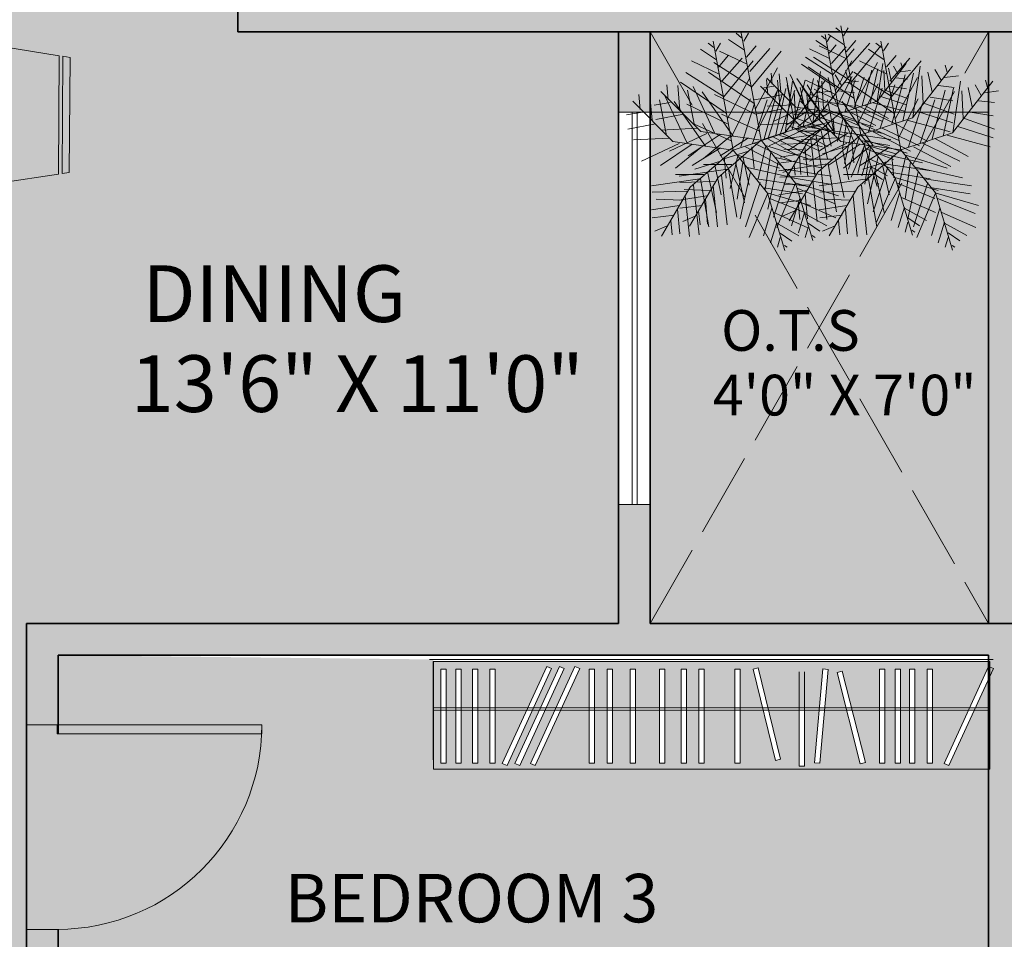
# Model space of a CAD drawing. Units: inches. Extents: x 1316 to 1777, y 813 to 1650.
# Tile 15 of 22: x 1567 to 1706, y 1237 to 1367. Entities that reach past the tile are written whole.
import ezdxf

# ---------------------------------------------------------------- set-up
doc = ezdxf.new("R2010")
doc.units = ezdxf.units.IN
doc.header["$MEASUREMENT"] = 0
doc.linetypes.add('ACAD_ISO02W100', pattern=[15, 12, -3])
for name, color, linetype, lineweight in [('A-AREA-IDEN', 7, 'Continuous', 18), ('A-DOOR', 4, 'Continuous', 18), ('A-DOOR-PATT', 253, 'Continuous', 13), ('A-FLOR-CASE-PATT', 252, 'Continuous', 13), ('A-FLOR-OPEN', 8, 'ACAD_ISO02W100', 13), ('A-FURN-PATT', 23, 'Continuous', 13), ('A-WALL-PATT', 250, 'Continuous', 13), ('closet', 23, 'Continuous', 18), ('furniture', 23, 'Continuous', 18), ('greenary', 106, 'Continuous', 13), ('L-HRDS', 8, 'Continuous', 18), ('L-HRDS-PATT', 252, 'Continuous', 13), ('L-PLNT-PATT', 74, 'Continuous', 13), ('walls', 250, 'Continuous', 35), ('windows', 141, 'Continuous', 18)]:
    doc.layers.add(name, color=color, linetype=linetype, lineweight=lineweight)
doc.layers.add('A-FLOR-PATT', color=254, linetype='Continuous', lineweight=13, true_color=0xfeeab9)
doc.styles.get("Standard").update_dxf_attribs({"font": 'arial.ttf'})

# ---------------------------------------------------------------- blocks, each defined once
blk = doc.blocks.new('*U15')
for p, q in [((0, 0), (0, -6)), ((40, 0), (40, -6))]:
    blk.add_line(p, q)
blk.add_lwpolyline([(0, 0), (0, 40), (1.75, 40), (1.75, 0)], close=True)
blk.add_arc((0, 0), 40, 0, 90)
blk = doc.blocks.new('Dining Set - 36 x 72 in.')
for p, q in [((-22, 27.5), (-22.1562, 26.50042)), ((-22, 27.5), (-6, 27.5)), ((-5.8437, 26.49966), (-6, 27.5)), ((6, 27.5), (5.8438, 26.50042)), ((6, 27.5), (22, 27.5)), ((22.1563, 26.49966), (22, 27.5)), ((-5.8416, 26.5), (-22.1534, 26.5)), ((22.1584, 26.5), (5.8466, 26.5)), ((-22.2343, 26.00059), (-23.4847, 17.99762)), ((-22.2304, 26), (-5.7608, 26)), ((-4.5152, 17.99762), (-5.7655, 25.99926)), ((5.7657, 26.00059), (4.5153, 17.99762)), ((5.7696, 26), (22.2392, 26)), ((23.4848, 17.99762), (22.2345, 25.99926)), ((36, 18), (-36, 18)), ((-36, 18), (-36, -18)), ((36, -18), (36, 18)), ((-44.0006, 8.23428), (-35.9976, 9.48474)), ((-44, 8.23041), (-44, -8.23915)), ((44.0006, 8.23428), (35.9976, 9.48474)), ((44, 8.23041), (44, -8.23915)), ((-45.5, 8), (-44.5004, 8.15617)), ((-45.5, 8), (-45.5, -8)), ((-44.5, -8.15843), (-44.5, 8.15338)), ((44.5, -8.15843), (44.5, 8.15338)), ((45.5, 8), (44.5005, 8.15617)), ((45.5, 8), (45.5, -8)), ((-44.4997, -8.15631), (-45.5, -8)), ((44.4997, -8.15631), (45.5, -8)), ((-35.9976, -9.48476), (-43.9993, -8.2345)), ((35.9976, -9.48476), (43.9993, -8.2345)), ((-36, -18), (36, -18)), ((-22.2343, -26.0006), (-23.4847, -17.99762)), ((-4.5152, -17.99762), (-5.7655, -25.99928)), ((5.7657, -26.0006), (4.5153, -17.99762)), ((23.4848, -17.99762), (22.2345, -25.99928)), ((-22.2304, -26), (-5.7608, -26)), ((5.7696, -26), (22.2392, -26)), ((-22, -27.5), (-22.1562, -26.50044)), ((-5.8416, -26.5), (-22.1534, -26.5)), ((-5.8437, -26.49967), (-6, -27.5)), ((6, -27.5), (5.8438, -26.50044)), ((22.1584, -26.5), (5.8466, -26.5)), ((22.1563, -26.49967), (22, -27.5)), ((-22, -27.5), (-6, -27.5)), ((6, -27.5), (22, -27.5))]:
    blk.add_line(p, q)
for points in [[(-36, 15), (-31.1772, 14.97754), (-26.8079, 14.91406), (-22.8538, 14.81543), (-19.276, 14.6875), (-16.0362, 14.53613), (-13.0957, 14.36718), (-10.4159, 14.18652), (-7.9583, 14), (-5.6904, 13.81315), (-3.6035, 13.63021), (-1.6954, 13.45508), (0.0365, 13.29166), (1.5945, 13.14388), (2.9811, 13.01562), (4.1988, 12.9108), (5.25, 12.83333), (6.1393, 12.78613), (6.8802, 12.76823), (7.4883, 12.77767), (7.9792, 12.8125), (8.3685, 12.87077), (8.6719, 12.95052), (8.9049, 13.0498), (9.0833, 13.16666), (9.2205, 13.29899), (9.3216, 13.44401), (9.3895, 13.59879), (9.4271, 13.76041), (9.4373, 13.92594), (9.4232, 14.09245), (9.3875, 14.257), (9.3333, 14.41666), (9.2638, 14.56917), (9.1836, 14.71484), (9.0975, 14.85465), (9.0104, 14.98958), (8.9272, 15.1206), (8.8529, 15.2487), (8.7922, 15.37483), (8.75, 15.5), (8.7305, 15.62467), (8.7344, 15.74739), (8.7617, 15.86621), (8.8125, 15.97916), (8.8867, 16.08431), (8.9844, 16.17968), (9.1055, 16.26334), (9.25, 16.33333), (9.4189, 16.38802), (9.6172, 16.42708), (9.8506, 16.45052), (10.125, 16.45833), (10.4463, 16.45052), (10.8203, 16.42708), (11.2529, 16.38802), (11.75, 16.33333), (12.3184, 16.26318), (12.9694, 16.17838), (13.7151, 16.07991), (14.5677, 15.96875), (15.5395, 15.84586), (16.6426, 15.71224), (17.8893, 15.56884), (19.2917, 15.41666), (20.859, 15.25667), (22.5879, 15.08984), (24.4721, 14.91715), (26.5052, 14.73958), (28.6809, 14.5581), (30.9929, 14.3737), (33.4347, 14.18733), (36, 14)], [(-36, 10), (-28.9766, 10.14274), (-23.1725, 10.20442), (-18.4241, 10.19775), (-14.5677, 10.13541), (-11.4399, 10.03011), (-8.877, 9.89453), (-6.7154, 9.74137), (-4.7917, 9.58333), (-2.9698, 9.43082), (-1.2246, 9.28515), (0.4415, 9.14534), (2.026, 9.01041), (3.5266, 8.87939), (4.9408, 8.7513), (6.266, 8.62516), (7.5, 8.5), (8.6411, 8.37549), (9.6914, 8.2539), (10.6538, 8.13818), (11.5312, 8.03125), (12.3267, 7.93603), (13.043, 7.85547), (13.6831, 7.79248), (14.25, 7.75), (14.7471, 7.7303), (15.1797, 7.73307), (15.5537, 7.75732), (15.875, 7.80208), (16.1494, 7.86637), (16.3828, 7.94922), (16.5811, 8.04964), (16.75, 8.16666), (16.8944, 8.29915), (17.0143, 8.44531), (17.1089, 8.60319), (17.1771, 8.77083), (17.218, 8.94629), (17.2305, 9.1276), (17.2137, 9.31282), (17.1667, 9.5), (17.0895, 9.6875), (16.987, 9.875), (16.8649, 10.0625), (16.7292, 10.25), (16.5856, 10.4375), (16.4401, 10.625), (16.2985, 10.8125), (16.1667, 11), (16.05, 11.18733), (15.9518, 11.3737), (15.8752, 11.5581), (15.8229, 11.73958), (15.798, 11.91715), (15.8034, 12.08984), (15.842, 12.25667), (15.9167, 12.41666), (16.0295, 12.56836), (16.1784, 12.70833), (16.3605, 12.83268), (16.5729, 12.9375), (16.8127, 13.01888), (17.0768, 13.07291), (17.3625, 13.0957), (17.6667, 13.08333), (17.9894, 13.03312), (18.3418, 12.94726), (18.7382, 12.82918), (19.1927, 12.68229), (19.7195, 12.51001), (20.3327, 12.31575), (21.0465, 12.10294), (21.875, 11.875), (22.8357, 11.63354), (23.959, 11.37304), (25.2786, 11.08618), (26.8282, 10.76562), (28.6414, 10.40405), (30.752, 9.99414), (33.1936, 9.52856), (36, 9)], [(-36, 5.5), (-30.7157, 5.3348), (-26.069, 5.20963), (-21.9946, 5.11767), (-18.4271, 5.05208), (-15.3009, 5.00602), (-12.5508, 4.97265), (-10.1112, 4.94515), (-7.9167, 4.91666), (-5.909, 4.88167), (-4.0586, 4.83984), (-2.3429, 4.79215), (-0.7396, 4.73958), (0.7739, 4.6831), (2.22, 4.6237), (3.6213, 4.56233), (5, 4.5), (6.373, 4.43782), (7.7344, 4.3776), (9.0723, 4.32129), (10.375, 4.27083), (11.6309, 4.22819), (12.8281, 4.19531), (13.9551, 4.17415), (15, 4.16666), (15.954, 4.17448), (16.819, 4.19791), (17.6001, 4.23698), (18.3021, 4.29166), (18.9299, 4.36198), (19.4883, 4.44791), (19.9823, 4.54948), (20.4167, 4.66666), (20.7969, 4.79899), (21.1302, 4.94401), (21.4245, 5.09879), (21.6875, 5.26041), (21.9271, 5.42594), (22.1511, 5.59245), (22.3672, 5.757), (22.5834, 5.91666), (22.8065, 6.06868), (23.0404, 6.21093), (23.2879, 6.34147), (23.5521, 6.45833), (23.8358, 6.55957), (24.142, 6.64323), (24.4735, 6.70735), (24.8334, 6.75), (25.2235, 6.76969), (25.642, 6.76692), (26.0858, 6.74267), (26.5521, 6.69791), (27.0379, 6.63362), (27.5404, 6.55078), (28.0565, 6.45036), (28.5834, 6.33333), (29.1242, 6.19987), (29.7071, 6.04687), (30.3661, 5.87044), (31.1354, 5.66666), (32.0493, 5.43164), (33.142, 5.16146), (34.4475, 4.85221), (36, 4.5)], [(-36, -1), (-30.7915, -0.6591), (-26.0195, -0.38216), (-21.6519, -0.16284), (-17.6563, 0.00521), (-14.0005, 0.12833), (-10.6523, 0.21289), (-7.5796, 0.26522), (-4.75, 0.29166), (-2.134, 0.29793), (0.2878, 0.28711), (2.5317, 0.26163), (4.6146, 0.22396), (6.5529, 0.17651), (8.3633, 0.12174), (10.0623, 0.06209), (11.6667, 0), (13.1899, -0.06201), (14.6341, -0.1211), (15.9982, -0.17432), (17.2813, -0.21875), (18.4823, -0.25147), (19.6003, -0.26953), (20.6343, -0.27002), (21.5834, -0.25), (22.4481, -0.20768), (23.2357, -0.14584), (23.9549, -0.06836), (24.6146, 0.02083), (25.2235, 0.11784), (25.7904, 0.21875), (26.3241, 0.31966), (26.8334, 0.41666), (27.3265, 0.50618), (27.8099, 0.58593), (28.2894, 0.65397), (28.7709, 0.70833), (29.2601, 0.74707), (29.763, 0.76823), (30.2855, 0.76985), (30.8334, 0.75), (31.4088, 0.70784), (31.9994, 0.64713), (32.589, 0.57275), (33.1615, 0.48958), (33.7008, 0.4025), (34.1908, 0.3164), (34.6153, 0.23616), (34.9584, 0.16666), (35.2099, 0.11165), (35.3848, 0.07031), (35.504, 0.04069), (35.5886, 0.02083), (35.6594, 0.00879), (35.7377, 0.0026), (35.8442, 0.00032), (36, 0)], [(-36, -6.5), (-27.1843, -6.31267), (-20.084, -6.1263), (-14.469, -5.9419), (-10.1094, -5.76042), (-6.7752, -5.58285), (-4.2363, -5.41016), (-2.2629, -5.24333), (-0.625, -5.08334), (0.8708, -4.93099), (2.2715, -4.78646), (3.5872, -4.64974), (4.8281, -4.52084), (6.0046, -4.39974), (7.127, -4.28646), (8.2053, -4.18099), (9.25, -4.08334), (10.2705, -3.99382), (11.2734, -3.91407), (12.2647, -3.84603), (13.25, -3.79167), (14.2354, -3.75293), (15.2266, -3.73177), (16.2295, -3.73015), (17.25, -3.75), (18.2912, -3.79248), (19.3451, -3.85547), (20.4009, -3.93604), (21.4479, -4.03125), (22.4754, -4.13819), (23.4727, -4.25391), (24.4289, -4.37549), (25.3334, -4.5), (26.1785, -4.62492), (26.9694, -4.74935), (27.7145, -4.87281), (28.4219, -4.99479), (29.1, -5.11483), (29.7572, -5.23242), (30.4016, -5.34709), (31.0417, -5.45834), (31.6837, -5.56437), (32.3262, -5.65821), (32.9658, -5.73153), (33.599, -5.77604), (34.2224, -5.78345), (34.8327, -5.74545), (35.4264, -5.65373), (36, -5.5)], [(-36, -10), (-26.4022, -9.81299), (-18.4675, -9.62891), (-11.9839, -9.45069), (-6.7396, -9.28125), (-2.5226, -9.12354), (0.8789, -8.98047), (3.6769, -8.85498), (6.0833, -8.75), (8.2767, -8.66765), (10.3021, -8.60677), (12.1712, -8.56543), (13.8958, -8.54167), (15.4876, -8.53353), (16.9583, -8.53907), (18.3197, -8.55632), (19.5834, -8.58334), (20.7616, -8.61841), (21.8685, -8.66081), (22.9188, -8.71004), (23.9271, -8.76563), (24.9081, -8.82707), (25.8763, -8.89388), (26.8465, -8.96558), (27.8334, -9.04167), (28.8474, -9.12118), (29.8828, -9.20117), (30.93, -9.27824), (31.9792, -9.34896), (33.0205, -9.40991), (34.0443, -9.45768), (35.0407, -9.48885), (36, -9.5)], [(-36, -14.5), (-30.0881, -14.33513), (-25.0332, -14.21224), (-20.7312, -14.12647), (-17.0781, -14.07292), (-13.97, -14.04671), (-11.3027, -14.04297), (-8.9724, -14.05681), (-6.875, -14.08334), (-4.9224, -14.11833), (-3.0905, -14.16016), (-1.3709, -14.20785), (0.2448, -14.26042), (1.7647, -14.3169), (3.1973, -14.3763), (4.5507, -14.43767), (5.8333, -14.5), (7.0554, -14.5621), (8.235, -14.62175), (9.3922, -14.67652), (10.5469, -14.72396), (11.7192, -14.76164), (12.929, -14.78711), (14.1965, -14.79794), (15.5417, -14.79167), (16.9933, -14.76424), (18.6152, -14.70508), (20.4804, -14.60197), (22.6615, -14.44271), (25.2312, -14.21509), (28.2624, -13.9069), (31.8277, -13.50594), (36, -13)]]:
    blk.add_lwpolyline(points)
blk = doc.blocks.new('dining area')
at = {"layer": 'furniture', "xscale": 0.6659924291999282, "yscale": 0.6659924291999282, "zscale": 0.6659924291999282, "rotation": 90}
blk.add_blockref('Dining Set - 36 x 72 in.', (-0.439, 20.507), dxfattribs=at)
blk = doc.blocks.new('*U13')
for p, q in [((0, 0), (-10.5, 57)), ((-8.737, 47.138), (-17.069, 52.711)), ((-10.186, 53.64), (-13.084, 55.962)), ((-9.099, 51.782), (-6.563, 55.962)), ((-7.288, 39.707), (-21.778, 46.673)), ((-7.65, 43.423), (-2.578, 49.46)), ((-5.839, 35.992), (4.667, 48.067)), ((-5.114, 27.632), (10.463, 46.673)), ((-5.114, 28.097), (-24.676, 40.636)), ((-2.941, 16.486), (8.652, 37.85)), ((44.153, 36.456), (45.239, 32.741)), ((-3.665, 19.273), (-27.574, 35.527)), ((16.259, 5.805), (23.142, 31.348)), ((22.055, 7.198), (27.489, 32.277)), ((27, 9), (48, 36)), ((27.127, 9.056), (31.112, 35.992)), ((35.096, 32.741), (37.27, 22.524)), ((38.719, 34.134), (41.979, 28.561)), ((-48.585, 21.131), (-49.309, 29.026)), ((-43.513, 28.561), (-42.427, 15.558)), ((-38.442, 26.239), (-34.819, 7.663)), ((-35.544, 28.097), (-24.314, 3.947)), ((-1.129, 6.734), (9.014, 26.704)), ((10.101, 3.483), (17.708, 26.239)), ((31.836, 30.883), (32.561, 16.486)), ((40.53, 25.775), (48.862, 24.846)), ((43.791, 29.954), (51.036, 30.883)), ((-31.5, 4.5), (-52.5, 25.5)), ((-14.533, 2.09), (-30.834, 25.31)), ((-24.314, 23.917), (-2.941, 13.7)), ((3.942, 1.625), (11.187, 24.381)), ((-47.498, 19.737), (-55.83, 18.344)), ((33.285, 16.486), (48.862, 10.913)), ((36.183, 19.737), (48.137, 17.88)), ((-40.615, 13.7), (-55.105, 10.913)), ((-20.691, 13.7), (-1.129, 4.876)), ((29.662, 12.307), (48.137, 6.269)), ((-33.37, 6.269), (-52.207, 5.34)), ((0, 0), (27, 9)), ((18.07, 5.805), (35.096, -3.483)), ((24.229, 7.663), (46.688, 1.625)), ((-28.299, 3.483), (-47.86, -5.805)), ((-21.416, 3.018), (-38.079, -8.128)), ((0, 0), (-31.5, 4.5)), ((-15.982, 2.09), (-30.11, -9.521)), ((0, 0), (-22.5, -19.5)), ((-6.563, 1.161), (-21.416, -8.128)), ((0, 0), (18, -22.5)), ((6.478, 1.625), (26.04, -8.592)), ((11.187, 3.483), (30.749, -5.805)), ((-4.752, -3.483), (-3.665, -14.629)), ((2.493, -3.019), (-1.491, -20.202)), ((1.769, -2.555), (24.229, -9.521)), ((-6.563, -5.805), (-19.967, -9.985)), ((-9.461, -8.592), (-6.201, -23.453)), ((5.029, -6.27), (2.131, -25.775)), ((7.565, -9.056), (32.198, -14.629)), ((-17.431, -15.094), (-42.789, -18.809)), ((-15.257, -12.772), (-30.11, -12.772)), ((-17.069, -15.094), (-12.721, -40.172)), ((-13.446, -11.378), (-8.737, -32.741)), ((9.014, -11.378), (3.58, -35.992)), ((12.274, -15.094), (36.907, -18.809)), ((-22.5, -19.5), (-37.5, -45)), ((-20.691, -18.345), (-17.793, -44.352)), ((14.085, -16.951), (6.478, -40.172)), ((16.259, -19.738), (36.183, -22.989)), ((-24.314, -21.596), (-42.427, -22.06)), ((-25.038, -23.918), (-22.865, -45.281)), ((18.07, -22.524), (8.289, -45.745)), ((18, -22.5), (27, -52.5)), ((18.433, -22.524), (40.53, -29.026)), ((19.157, -25.311), (38.719, -33.206)), ((-28.299, -29.026), (-42.789, -31.348)), ((-26.849, -26.24), (-40.253, -25.775)), ((-29.023, -30.884), (-27.936, -43.887)), ((20.244, -30.419), (15.897, -44.816)), ((-30.834, -34.135), (-42.427, -35.528)), ((21.331, -32.741), (39.081, -40.636)), ((-34.457, -39.708), (-40.978, -42.494)), ((-32.646, -36.921), (-31.921, -44.352)), ((22.78, -37.85), (19.519, -48.532)), ((22.78, -38.314), (34.372, -44.816)), ((24.591, -45.745), (23.142, -50.854)), ((24.591, -43.423), (30.749, -47.603)), ((26.764, -49.925), (28.213, -50.854))]:
    blk.add_line(p, q)
blk = doc.blocks.new('closet')
at = {"layer": 'closet'}
for p, q in [((-0.71, -5.58), (5.59, 8.19)), ((-0.23, 7.39), (-0.23, -6.57)), ((6.27, 7.88), (-0.04, -5.89)), ((5.59, 8.19), (6.27, 7.88)), ((7.92, 7.84), (8.68, 7.84)), ((7.92, 7.84), (7.92, -5.51)), ((8.68, 7.84), (8.68, -5.51)), ((10.44, 7.84), (11.2, 7.84)), ((10.44, 7.84), (10.44, -5.51)), ((11.2, 7.84), (11.2, -5.51)), ((12.45, 7.84), (13.21, 7.84)), ((12.45, 7.84), (12.45, -5.51)), ((13.21, 7.84), (13.21, -5.51)), ((14.71, 7.84), (15.47, 7.84)), ((14.71, 7.84), (14.71, -5.51)), ((15.47, 7.84), (15.47, -5.51)), ((17.44, 7.75), (18.17, 7.93)), ((17.44, 7.75), (20.73, -5.2)), ((18.17, 7.93), (21.46, -5.01)), ((23.92, 7.84), (22.75, -5.46)), ((24.67, 7.78), (23.51, -5.53)), ((23.92, 7.84), (24.67, 7.78)), ((26.09, 8.25), (26.09, -5.1)), ((26.84, 8.25), (26.84, -5.1)), ((29.49, 7.29), (32.64, -5.69)), ((30.22, 7.46), (33.37, -5.51)), ((35.23, 7.84), (35.23, -5.51)), ((35.99, 7.84), (35.99, -5.51)), ((40.33, 7.84), (40.33, -5.51)), ((41.08, 7.84), (41.08, -5.51)), ((42.85, 7.84), (42.85, -5.51)), ((43.61, 7.84), (43.61, -5.51)), ((45.9, 7.84), (45.9, -5.51)), ((46.65, 7.84), (46.65, -5.51)), ((50.07, 7.84), (50.07, -5.51)), ((50.82, 7.84), (50.82, -5.51)), ((53.32, 7.84), (53.32, -5.51)), ((54.08, 7.84), (54.08, -5.51)), ((55.9, 7.84), (55.9, -5.51)), ((56.65, 7.84), (56.65, -5.51)), ((57.99, -5.58), (64.3, 8.19)), ((64.97, 7.88), (58.67, -5.89)), ((60.19, -5.58), (66.49, 8.19)), ((67.17, 7.88), (60.87, -5.89)), ((62, -5.58), (68.3, 8.19)), ((68.98, 7.88), (62.67, -5.89)), ((69.96, 7.84), (69.96, -5.51)), ((70.72, 7.84), (70.72, -5.51)), ((72.43, 7.84), (72.43, -5.51)), ((73.19, 7.84), (73.19, -5.51)), ((74.82, 7.84), (74.82, -5.51)), ((75.57, 7.84), (75.57, -5.51)), ((76.94, 7.84), (76.94, -5.51)), ((77.69, 7.84), (77.69, -5.51)), ((56.23, 0.33), (0, 0.33)), ((56.2, 0), (0, 0)), ((56.2, 0), (78.76, 0)), ((56.23, 0.33), (78.76, 0.33)), ((-0.04, -5.89), (-0.71, -5.58)), ((21.46, -5.01), (20.73, -5.2)), ((23.51, -5.53), (22.75, -5.46)), ((33.37, -5.51), (32.64, -5.69)), ((35.99, -5.51), (35.23, -5.51)), ((41.08, -5.51), (40.33, -5.51)), ((43.61, -5.51), (42.85, -5.51)), ((46.65, -5.51), (45.9, -5.51)), ((50.82, -5.51), (50.07, -5.51)), ((54.08, -5.51), (53.32, -5.51)), ((56.65, -5.51), (55.9, -5.51)), ((58.67, -5.89), (57.99, -5.58)), ((60.87, -5.89), (60.19, -5.58)), ((62.67, -5.89), (62, -5.58)), ((70.72, -5.51), (69.96, -5.51)), ((73.19, -5.51), (72.43, -5.51)), ((75.57, -5.51), (74.82, -5.51)), ((77.69, -5.51), (76.94, -5.51))]:
    blk.add_line(p, q, dxfattribs=at)
blk = doc.blocks.new('rotated closet')
at = {"layer": 'closet'}
for p, q in [((26.32, 0.86), (27.07, 0.86)), ((29.72, -0.11), (30.45, 0.07)), ((35.46, 0.45), (36.22, 0.45)), ((40.56, 0.45), (41.31, 0.45)), ((43.08, 0.45), (43.84, 0.45)), ((46.13, 0.45), (46.88, 0.45)), ((50.3, 0.45), (51.05, 0.45)), ((53.56, 0.45), (54.31, 0.45)), ((56.13, 0.45), (56.88, 0.45)), ((64.53, 0.8), (65.2, 0.49)), ((66.72, 0.8), (67.4, 0.49)), ((68.53, 0.8), (69.21, 0.49)), ((70.19, 0.45), (70.95, 0.45)), ((72.66, 0.45), (73.42, 0.45)), ((75.05, 0.45), (75.81, 0.45)), ((77.17, 0.45), (77.92, 0.45)), ((78.99, 0), (78.99, -13.96)), ((0, -13.96), (78.99, -13.96)), ((8.91, -12.91), (8.15, -12.91)), ((11.43, -12.91), (10.67, -12.91)), ((13.44, -12.91), (12.68, -12.91)), ((15.7, -12.91), (14.94, -12.91)), ((-0.46, -14.27), (79.54, -14.27))]:
    blk.add_line(p, q, dxfattribs=at)
blk.add_blockref('closet', (0.23, -7.39), dxfattribs=at)
blk = doc.blocks.new('WARDROBE-80')
for p, q in [((80, 15.57), (0, 15.57)), ((80, 15.57), (0, 15.57)), ((80, 15.57), (0, 15.57)), ((0.56, 15.25), (0.56, 0.44)), ((79.54, 15.25), (0.56, 15.25)), ((79.54, 15.25), (2.2, 15.25)), ((79.54, 0), (79.54, 15.25)), ((0.56, 0), (0.56, 0.44)), ((79.54, 0), (0.56, 0))]:
    blk.add_line(p, q)
at = {"rotation": 179.9999999959433}
blk.add_blockref('rotated closet', (79.54, 1.29), dxfattribs=at)

msp = doc.modelspace()

# ---------------------------------------------------------------- hatches: boundary and pattern name
at = {"layer": 'A-DOOR-PATT'}
h = msp.add_hatch(color=256, dxfattribs=at)
h.dxf.hatch_style = 1
h.paths.add_polyline_path([(1601.07, 1266.995), (1572.173, 1266.995), (1572.173, 1265.725), (1601.042, 1265.725, 0.0109414)])
h.paths.add_polyline_path([(1574.225, 1069.579, 0.0109414), (1572.764, 1069.547), (1572.764, 1040.173), (1574.225, 1040.173)])
h.paths.add_polyline_path([(1574.225, 1040.173), (1572.764, 1040.173), (1572.764, 1036.182), (1574.225, 1036.182)])
at = {"layer": 'A-FLOR-CASE-PATT'}
h = msp.add_hatch(color=256, dxfattribs=at)
h.dxf.hatch_style = 1
h.paths.add_polyline_path([(1647.51, 1269.064), (1643.462, 1269.064), (1639.865, 1261.207), (1639.189, 1261.517), (1642.645, 1269.064), (1641.267, 1269.064), (1637.669, 1261.207), (1636.994, 1261.517), (1640.449, 1269.064), (1639.457, 1269.064), (1635.86, 1261.207), (1635.184, 1261.517), (1638.64, 1269.064), (1634.199, 1269.064), (1634.199, 1261.557), (1633.442, 1261.557), (1633.442, 1269.064), (1631.734, 1269.064), (1631.734, 1261.557), (1630.977, 1261.557), (1630.977, 1269.064), (1629.345, 1269.064), (1629.345, 1261.557), (1628.588, 1261.557), (1628.588, 1269.064), (1627.226, 1269.064), (1627.226, 1261.557), (1626.47, 1261.557), (1626.47, 1269.064), (1625.405, 1269.064), (1625.405, 1262.004), (1625.405, 1261.154), (1625.405, 1260.711), (1704.173, 1260.711), (1704.173, 1269.064), (1702.168, 1269.064), (1698.57, 1261.207), (1697.895, 1261.517), (1701.35, 1269.064), (1696.241, 1269.064), (1696.241, 1261.557), (1695.484, 1261.557), (1695.484, 1269.064), (1693.719, 1269.064), (1693.719, 1261.557), (1692.963, 1261.557), (1692.963, 1269.064), (1691.713, 1269.064), (1691.713, 1261.557), (1690.957, 1261.557), (1690.957, 1269.064), (1689.451, 1269.064), (1689.451, 1261.557), (1688.694, 1261.557), (1688.694, 1269.064), (1684.84, 1269.064), (1686.726, 1261.65), (1685.993, 1261.464), (1684.06, 1269.064), (1680.901, 1269.064), (1680.244, 1261.557), (1679.49, 1261.623), (1680.141, 1269.064), (1678.076, 1269.064), (1678.076, 1261.145), (1677.32, 1261.145), (1677.32, 1269.064), (1672.99, 1269.064), (1674.677, 1262.112), (1673.942, 1261.934), (1672.211, 1269.064), (1668.933, 1269.064), (1668.933, 1261.557), (1668.177, 1261.557), (1668.177, 1269.064), (1663.836, 1269.064), (1663.836, 1261.557), (1663.08, 1261.557), (1663.08, 1269.064), (1661.314, 1269.064), (1661.314, 1261.557), (1660.557, 1261.557), (1660.557, 1269.064), (1658.266, 1269.064), (1658.266, 1261.557), (1657.51, 1261.557), (1657.51, 1269.064), (1654.096, 1269.064), (1654.096, 1261.557), (1653.339, 1261.557), (1653.339, 1269.064), (1650.838, 1269.064), (1650.838, 1261.557), (1650.081, 1261.557), (1650.081, 1269.064), (1648.266, 1269.064), (1648.266, 1261.557), (1647.51, 1261.557)])
h.paths.add_polyline_path([(1641.488, 1275.285), (1642.164, 1274.975), (1639.61, 1269.398), (1640.602, 1269.398), (1643.297, 1275.285), (1643.973, 1274.975), (1641.42, 1269.398), (1642.798, 1269.398), (1645.493, 1275.285), (1646.169, 1274.975), (1643.616, 1269.398), (1647.51, 1269.398), (1647.51, 1274.913), (1648.266, 1274.913), (1648.266, 1269.398), (1650.081, 1269.398), (1650.081, 1274.913), (1650.838, 1274.913), (1650.838, 1269.398), (1653.339, 1269.398), (1653.339, 1274.913), (1654.096, 1274.913), (1654.096, 1269.398), (1657.51, 1269.398), (1657.51, 1274.913), (1658.266, 1274.913), (1658.266, 1269.398), (1660.557, 1269.398), (1660.557, 1274.913), (1661.314, 1274.913), (1661.314, 1269.398), (1663.08, 1269.398), (1663.08, 1274.913), (1663.836, 1274.913), (1663.836, 1269.398), (1668.177, 1269.398), (1668.177, 1274.913), (1668.933, 1274.913), (1668.933, 1269.398), (1672.13, 1269.398), (1670.791, 1274.913), (1671.526, 1275.092), (1672.908, 1269.398), (1680.17, 1269.398), (1680.654, 1274.929), (1681.408, 1274.863), (1680.93, 1269.398), (1683.974, 1269.398), (1682.7, 1274.408), (1683.434, 1274.595), (1684.755, 1269.398), (1688.694, 1269.398), (1688.694, 1274.913), (1689.451, 1274.913), (1689.451, 1269.398), (1690.957, 1269.398), (1690.957, 1274.913), (1691.713, 1274.913), (1691.713, 1269.398), (1692.963, 1269.398), (1692.963, 1274.913), (1693.719, 1274.913), (1693.719, 1269.398), (1695.484, 1269.398), (1695.484, 1274.913), (1696.241, 1274.913), (1696.241, 1269.398), (1701.503, 1269.398), (1704.173, 1275.229), (1704.173, 1275.964), (1625.405, 1275.964), (1625.405, 1269.398), (1626.47, 1269.398), (1626.47, 1274.913), (1627.226, 1274.913), (1627.226, 1269.398), (1628.588, 1269.398), (1628.588, 1274.913), (1629.345, 1274.913), (1629.345, 1269.398), (1630.977, 1269.398), (1630.977, 1274.913), (1631.734, 1274.913), (1631.734, 1269.398), (1633.442, 1269.398), (1633.442, 1274.913), (1634.199, 1274.913), (1634.199, 1269.398), (1638.793, 1269.398)])
h.paths.add_polyline_path([(1704.173, 1273.444), (1702.321, 1269.398), (1704.173, 1269.398)], flags=0)
h = msp.add_hatch(color=256, dxfattribs=at)
h.dxf.hatch_style = 1
h.paths.add_polyline_path([(1704.173, 1273.444), (1702.321, 1269.398), (1704.173, 1269.398)])
at = {"layer": 'A-FLOR-PATT'}
h = msp.add_hatch(color=256, dxfattribs=at)
h.dxf.hatch_style = 1
h.paths.add_polyline_path([(1567.673, 1281.369), (1651.673, 1281.369), (1651.673, 1365.369), (1597.673, 1365.369), (1597.673, 1429.869), (1570.345, 1429.869), (1570.345, 1471.869), (1510.345, 1471.869), (1510.345, 1429.869), (1444.564, 1429.869), (1444.564, 1322.882), (1444.564, 1300.088), (1510.564, 1300.088), (1510.564, 1295.094), (1510.564, 1240.869), (1386.064, 1240.869), (1386.064, 1171.185), (1400.961, 1171.185), (1400.961, 1106.742), (1386.064, 1106.742), (1386.064, 1072.869), (1510.564, 1072.869), (1510.564, 1040.173), (1541.068, 1040.173, -0.367085), (1572.764, 1069.547), (1572.764, 1069.579), (1574.225, 1069.579), (1574.225, 1040.173), (1616.037, 1040.173), (1616.037, 1086.627), (1616.037, 1103.705), (1613.066, 1105.235), (1616.037, 1106.686), (1616.037, 1123.869), (1567.673, 1123.869)])
h.paths.add_polyline_path([(1508.987, 1198.018), (1511.117, 1198.018), (1511.117, 1200.148), (1532.595, 1200.148), (1532.595, 1198.018), (1534.725, 1198.018), (1534.725, 1176.008), (1530.465, 1176.008), (1530.465, 1176.718), (1513.247, 1176.718), (1513.247, 1176.008), (1508.987, 1176.008)], flags=16)
h.paths.add_polyline_path([(1505.979, 1151.315), (1521.504, 1151.315), (1521.504, 1123.623), (1505.979, 1123.623)], flags=16)
h.paths.add_polyline_path([(1507.734, 1150.101, -1), (1506.932, 1150.101, -1)], flags=0)
h.paths.add_polyline_path([(1512.288, 1138.353), (1512.28, 1138.392), (1512.219, 1138.376)], flags=0)
h.paths.add_polyline_path([(1511.539, 1138.926), (1511.802, 1138.967), (1511.817, 1139.27), (1511.607, 1139.246)], flags=0)
h.paths.add_polyline_path([(1513.745, 1140.234), (1513.68, 1139.885), (1514.014, 1140.045), (1513.855, 1140.308)], flags=0)
h.paths.add_polyline_path([(1513.759, 1139.089), (1514.005, 1139.255), (1513.807, 1139.483), (1513.564, 1139.327)], flags=0)
h.paths.add_polyline_path([(1514.219, 1138.385), (1514.336, 1138.33), (1514.544, 1138.32), (1514.802, 1138.874), (1514.451, 1138.716)], flags=0)
h.paths.add_polyline_path([(1514.577, 1137.439), (1514.573, 1137.4), (1514.699, 1137.4), (1514.696, 1137.402)], flags=0)
h.paths.add_polyline_path([(1512.26, 1136.199), (1512.199, 1136.399), (1512.032, 1136.325), (1512.095, 1136.101), (1512.257, 1136.192)], flags=0)
h.paths.add_polyline_path([(1512.644, 1137.274), (1512.356, 1137.23), (1512.432, 1137.049), (1512.703, 1137.093)], flags=0)
h.paths.add_polyline_path([(1513.049, 1137.593), (1512.979, 1137.8), (1512.843, 1137.757), (1512.887, 1137.556)], flags=0)
h.paths.add_polyline_path([(1513.269, 1138.556), (1513.571, 1137.962), (1513.459, 1136.814), (1513.212, 1137.878), (1513.032, 1138.443)], flags=0)
h.paths.add_polyline_path([(1514.891, 1136.377), (1514.696, 1136.401), (1514.683, 1136.246), (1514.87, 1136.165)], flags=0)
h.paths.add_polyline_path([(1514.142, 1137.293), (1514.047, 1136.743), (1514.27, 1136.751), (1514.328, 1137.265)], flags=0)
h.paths.add_polyline_path([(1515.362, 1138.976), (1515.334, 1138.638), (1515.596, 1138.588), (1515.627, 1138.932)], flags=0)
h.paths.add_polyline_path([(1537.285, 1177.912), (1537.995, 1177.912), (1537.995, 1195.13), (1537.285, 1195.13), (1537.285, 1199.39), (1559.295, 1199.39), (1559.295, 1197.26), (1561.425, 1197.26), (1561.425, 1175.782), (1559.295, 1175.782), (1559.295, 1173.652), (1559.379, 1173.652), (1559.379, 1171.514), (1561.517, 1171.514), (1561.517, 1098.819), (1559.379, 1098.819), (1559.379, 1096.68), (1537.285, 1096.68), (1537.285, 1100.957), (1537.997, 1100.957), (1537.997, 1169.376), (1537.285, 1169.376), (1537.285, 1173.652)], flags=16)
h.paths.add_polyline_path([(1518.623, 1345.565), (1519.133, 1345.48), (1519.133, 1345.485), (1518.623, 1345.567)], flags=16)
h.paths.add_polyline_path([(1518.798, 1374.15), (1519.308, 1374.064), (1519.308, 1374.069), (1518.798, 1374.152)], flags=16)
h.paths.add_polyline_path([(1537.764, 1413.501), (1537.678, 1412.991), (1537.683, 1412.991), (1537.766, 1413.501)], flags=16)
h.paths.add_polyline_path([(1572.905, 1373.821), (1573.927, 1373.975), (1574.027, 1390.309), (1573.007, 1390.475), (1573.007, 1390.475)], flags=16)
h.paths.add_polyline_path([(1572.73, 1345.237), (1573.752, 1345.39), (1573.852, 1361.724), (1572.832, 1361.89), (1572.832, 1361.89)], flags=16)
h.paths.add_polyline_path([(1537.211, 1322.643), (1537.364, 1321.621), (1553.698, 1321.521), (1553.864, 1322.541)], flags=16)
h.paths.add_polyline_path([(1535.908, 1331.328), (1527.214, 1331.382), (1527.664, 1404.885), (1564.416, 1404.66), (1563.966, 1331.157), (1555.273, 1331.21), (1553.947, 1323.051), (1537.134, 1323.154)], flags=16)
h.paths.add_polyline_path([(1536.15, 1336.503), (1536.235, 1337.572), (1536.323, 1338.628), (1536.411, 1339.663), (1536.495, 1340.67), (1536.574, 1341.66), (1536.648, 1342.648), (1536.717, 1343.649), (1536.78, 1344.678), (1536.837, 1345.75), (1536.913, 1347.475), (1536.93, 1348.082), (1536.867, 1346.314), (1536.754, 1344.188), (1536.619, 1342.219), (1536.495, 1340.67), (1536.411, 1339.663), (1536.323, 1338.628), (1536.235, 1337.572), (1536.15, 1336.503), (1536.071, 1335.432), (1536.002, 1334.37), (1535.917, 1332.754), (1535.909, 1332.308), (1535.964, 1333.78), (1536.071, 1335.432)], flags=0)
h.paths.add_polyline_path([(1540.412, 1338.345), (1540.539, 1339.037), (1540.667, 1339.758), (1540.798, 1340.518), (1540.93, 1341.325), (1541.063, 1342.187), (1541.196, 1343.109), (1541.326, 1344.085), (1541.45, 1345.102), (1541.566, 1346.15), (1541.669, 1347.219), (1541.758, 1348.296), (1541.829, 1349.371), (1541.879, 1350.434), (1541.906, 1351.476), (1541.91, 1352.5), (1541.895, 1353.512), (1541.861, 1354.518), (1541.812, 1355.524), (1541.749, 1356.537), (1541.674, 1357.561), (1541.551, 1359.062), (1541.495, 1359.67), (1541.589, 1358.603), (1541.721, 1356.977), (1541.846, 1354.98), (1541.912, 1352.982), (1541.903, 1350.951), (1541.806, 1348.87), (1541.628, 1346.713), (1541.396, 1344.612), (1541.135, 1342.656), (1540.872, 1340.947), (1540.617, 1339.466), (1540.412, 1338.345), (1540.288, 1337.675), (1540.166, 1337.018), (1540.049, 1336.365), (1539.937, 1335.71), (1539.837, 1335.055), (1539.758, 1334.403), (1539.709, 1333.756), (1539.697, 1333.12), (1539.751, 1332.162), (1539.822, 1331.89), (1539.691, 1332.775), (1539.714, 1334.035), (1539.867, 1335.303), (1540.085, 1336.577), (1540.288, 1337.675)], flags=0)
h.paths.add_polyline_path([(1545.599, 1331.584), (1545.601, 1331.617), (1545.614, 1331.689), (1545.737, 1332.197), (1545.767, 1332.332), (1545.84, 1332.681), (1545.925, 1333.114), (1546.016, 1333.614), (1546.108, 1334.164), (1546.196, 1334.748), (1546.276, 1335.349), (1546.342, 1335.952), (1546.388, 1336.539), (1546.412, 1337.098), (1546.414, 1337.632), (1546.395, 1338.145), (1546.359, 1338.645), (1546.306, 1339.137), (1546.24, 1339.627), (1546.161, 1340.121), (1546.073, 1340.625), (1545.888, 1341.63), (1545.718, 1342.621), (1545.547, 1343.945), (1545.432, 1345.534), (1545.404, 1347.402), (1545.418, 1348.013), (1545.411, 1346.957), (1545.425, 1345.988), (1545.463, 1345.105), (1545.521, 1344.301), (1545.596, 1343.566), (1545.683, 1342.892), (1545.778, 1342.27), (1545.877, 1341.691), (1545.977, 1341.145), (1546.133, 1340.297), (1546.327, 1339.075), (1546.434, 1337.615), (1546.377, 1336.279), (1546.246, 1335.079), (1546.032, 1333.665), (1545.84, 1332.681), (1545.767, 1332.332)], flags=0)
h.paths.add_polyline_path([(1551.803, 1337.656), (1551.963, 1338.25), (1552.102, 1338.801), (1552.225, 1339.338), (1552.331, 1339.865), (1552.418, 1340.377), (1552.487, 1340.873), (1552.536, 1341.348), (1552.563, 1341.801), (1552.569, 1342.228), (1552.551, 1342.627), (1552.51, 1342.995), (1552.446, 1343.333), (1552.363, 1343.646), (1552.261, 1343.937), (1552.144, 1344.207), (1552.012, 1344.461), (1551.868, 1344.7), (1551.746, 1344.882), (1550.887, 1346.052), (1550.428, 1347.126), (1550.183, 1348.353), (1550.048, 1349.632), (1549.978, 1351.224), (1549.974, 1353.141), (1549.989, 1353.748), (1549.975, 1352.682), (1549.977, 1351.708), (1549.996, 1350.825), (1550.031, 1350.027), (1550.082, 1349.31), (1550.15, 1348.669), (1550.234, 1348.098), (1550.335, 1347.593), (1550.452, 1347.149), (1550.584, 1346.76), (1550.73, 1346.419), (1550.887, 1346.117), (1551.05, 1345.848), (1551.217, 1345.602), (1551.386, 1345.372), (1551.553, 1345.151), (1552, 1344.537), (1552.454, 1343.495), (1552.591, 1342.266), (1552.509, 1340.905), (1552.246, 1339.367), (1551.925, 1338.101), (1551.619, 1336.984), (1551.406, 1336.2), (1551.01, 1334.699), (1550.877, 1334.155), (1551.264, 1335.677), (1551.619, 1336.984)], flags=0)
h.paths.add_polyline_path([(1558.642, 1348.348), (1558.795, 1348.811), (1558.918, 1349.215), (1559.008, 1349.575), (1559.061, 1349.904), (1559.076, 1350.214), (1559.054, 1350.506), (1559.001, 1350.776), (1558.919, 1351.021), (1558.814, 1351.239), (1558.688, 1351.425), (1558.546, 1351.578), (1558.392, 1351.694), (1558.229, 1351.772), (1558.059, 1351.812), (1557.882, 1351.819), (1557.701, 1351.794), (1557.515, 1351.742), (1557.327, 1351.665), (1557.136, 1351.566), (1556.944, 1351.448), (1556.752, 1351.315), (1556.742, 1351.307), (1556.175, 1350.878), (1555.982, 1350.741), (1555.79, 1350.618), (1555.103, 1350.248), (1554.019, 1350.696), (1553.658, 1351.734), (1553.592, 1352.861), (1553.705, 1354.248), (1553.753, 1354.657), (1553.685, 1354.004), (1553.638, 1353.425), (1553.615, 1352.918), (1553.615, 1352.476), (1553.637, 1352.094), (1553.681, 1351.766), (1553.745, 1351.485), (1553.828, 1351.246), (1553.929, 1351.043), (1554.048, 1350.87), (1554.182, 1350.722), (1554.33, 1350.599), (1554.491, 1350.501), (1554.662, 1350.43), (1554.841, 1350.388), (1555.026, 1350.374), (1555.215, 1350.39), (1555.406, 1350.437), (1555.598, 1350.514), (1555.79, 1350.618), (1555.982, 1350.741), (1556.175, 1350.878), (1556.367, 1351.024), (1556.559, 1351.171), (1556.752, 1351.315), (1556.944, 1351.448), (1557.136, 1351.566), (1557.327, 1351.665), (1558.043, 1351.957), (1558.894, 1351.316), (1559.137, 1350.09), (1558.886, 1349.087), (1558.642, 1348.348), (1558.463, 1347.812), (1558.261, 1347.187), (1558.039, 1346.459), (1557.677, 1345.175), (1557.549, 1344.636), (1557.909, 1346.03), (1558.329, 1347.408)], flags=0)
h.paths.add_polyline_path([(1562.145, 1353.919), (1562.25, 1354.68), (1562.341, 1355.344), (1562.416, 1355.924), (1562.475, 1356.431), (1562.518, 1356.872), (1562.544, 1357.254), (1562.554, 1357.582), (1562.548, 1357.862), (1562.525, 1358.1), (1562.486, 1358.303), (1562.432, 1358.476), (1562.361, 1358.624), (1562.277, 1358.748), (1562.18, 1358.848), (1562.073, 1358.925), (1561.958, 1358.977), (1561.837, 1359.006), (1561.711, 1359.011), (1561.584, 1358.992), (1561.456, 1358.949), (1561.342, 1358.895), (1560.78, 1358.554), (1560.631, 1358.473), (1560.474, 1358.403), (1560.311, 1358.348), (1559.637, 1358.207), (1558.973, 1358.904), (1558.816, 1360.002), (1558.804, 1361.236), (1558.83, 1361.674), (1558.807, 1360.917), (1558.813, 1360.297), (1558.845, 1359.795), (1558.902, 1359.397), (1558.982, 1359.087), (1559.082, 1358.849), (1559.2, 1358.666), (1559.334, 1358.525), (1559.482, 1358.421), (1559.639, 1358.351), (1559.804, 1358.311), (1559.973, 1358.3), (1560.143, 1358.313), (1560.311, 1358.348), (1560.474, 1358.403), (1560.631, 1358.473), (1560.78, 1358.554), (1560.923, 1358.641), (1561.061, 1358.729), (1561.196, 1358.813), (1561.382, 1358.92), (1561.342, 1358.895), (1561.972, 1359.194), (1562.536, 1358.367), (1562.56, 1357.311), (1562.455, 1356.226), (1562.323, 1355.206), (1562.145, 1353.919), (1562.026, 1353.049), (1561.815, 1351.457), (1561.752, 1350.933), (1561.948, 1352.479)], flags=0)
h.paths.add_polyline_path([(1572.764, 1069.547, 0.367085), (1541.068, 1040.173), (1572.764, 1040.173)], flags=17)
h.paths.add_polyline_path([(1572.764, 1040.173), (1541.068, 1040.173, 0.0299535), (1540.829, 1036.182), (1540.829, 1031.173), (1574.225, 1031.173), (1574.225, 1036.182), (1572.764, 1036.182)])
h = msp.add_hatch(color=256, dxfattribs=at)
h.dxf.hatch_style = 1
h.paths.add_polyline_path([(1704.173, 1260.711), (1625.405, 1260.711), (1625.405, 1261.154), (1625.405, 1276.279), (1624.85, 1276.279), (1572.173, 1276.869), (1572.173, 1266.995), (1601.07, 1266.995), (1601.07, 1265.725), (1601.042, 1265.725, -0.4000145), (1572.173, 1237.955), (1572.173, 1132.869), (1704.173, 1132.869)])
edge = h.paths.add_edge_path(flags=0)
edge.add_spline(control_points=[(1634.063, 1215.447), (1634.008, 1215.524), (1633.887, 1215.694), (1634.084, 1216.011), (1634.356, 1216.402), (1634.084, 1216.621), (1633.946, 1216.732)], knot_values=[0, 0, 0, 0, 0.3739943, 0.8243137, 1.461173, 2.1144513, 2.1144513, 2.1144513, 2.1144513], degree=3, periodic=0)
edge.add_spline(control_points=[(1633.711, 1215.447), (1633.656, 1215.524), (1633.535, 1215.694), (1633.732, 1216.011), (1634.005, 1216.402), (1633.732, 1216.621), (1633.594, 1216.732)], knot_values=[0, 0, 0, 0, 0.3739943, 0.8243137, 1.461173, 2.1144513, 2.1144513, 2.1144513, 2.1144513], degree=3, periodic=0)
edge = h.paths.add_edge_path(flags=16)
edge.add_line((1631.459, 1215.447), (1661.482, 1215.447))
edge.add_line((1661.482, 1215.447), (1661.482, 1208.307))
edge.add_line((1661.482, 1208.307), (1688.953, 1208.307))
edge.add_line((1688.953, 1208.307), (1688.837, 1220.405))
edge.add_line((1688.837, 1220.405), (1702.711, 1220.405))
edge.add_line((1702.711, 1220.405), (1702.827, 1208.307))
edge.add_line((1702.827, 1208.307), (1702.827, 1154.307))
edge.add_line((1702.827, 1154.307), (1702.944, 1142.208))
edge.add_line((1702.944, 1142.208), (1689.07, 1142.208))
edge.add_line((1689.07, 1142.208), (1688.953, 1154.307))
edge.add_line((1688.953, 1154.307), (1661.482, 1154.307))
edge.add_line((1661.482, 1154.307), (1661.482, 1143.444))
edge.add_line((1661.482, 1143.444), (1634.022, 1143.444))
edge.add_spline(control_points=[(1634.022, 1143.444), (1633.972, 1143.371), (1633.857, 1143.204), (1634.053, 1142.892), (1634.324, 1142.501), (1634.052, 1142.282), (1633.914, 1142.172)], knot_values=[0, 0, 0, 0, 0.3521435, 0.8024629, 1.4393222, 2.0926005, 2.0926005, 2.0926005, 2.0926005], degree=3, periodic=0)
edge.add_spline(control_points=[(1633.562, 1142.172), (1633.7, 1142.282), (1633.973, 1142.501), (1633.701, 1142.892), (1633.505, 1143.204), (1633.62, 1143.371), (1633.67, 1143.444)], knot_values=[0, 0, 0, 0, 0.6532783, 1.2901376, 1.740457, 2.0926005, 2.0926005, 2.0926005, 2.0926005], degree=3, periodic=0)
edge.add_line((1633.67, 1143.444), (1631.459, 1143.444))
edge.add_line((1631.459, 1143.444), (1631.459, 1215.447))
h.paths.add_polyline_path([(1691.549, 1164.108), (1691.597, 1164.173), (1691.597, 1202.209), (1699.757, 1202.209), (1699.757, 1186.386), (1691.597, 1186.386), (1691.597, 1179.931), (1699.757, 1179.931), (1699.757, 1164.108), (1691.549, 1164.108), (1684.365, 1154.365), (1684.365, 1164.108)], flags=0)
h.paths.add_polyline_path([(1691.424, 1214.03, -1), (1700.356, 1214.03, -1)], flags=0)
h.paths.add_polyline_path([(1691.541, 1147.932, -1), (1700.473, 1147.932, -1)], flags=0)
h.paths.add_polyline_path([(1601.042, 1265.725), (1572.029, 1265.725), (1572.029, 1266.995), (1567.673, 1266.995), (1567.673, 1237.955), (1572.029, 1237.955, 0.4014527)])
at = {"layer": 'A-FURN-PATT'}
h = msp.add_hatch(color=256, dxfattribs=at)
h.dxf.hatch_style = 1
h.paths.add_polyline_path([(1527.586, 1392.108), (1519.411, 1390.882), (1519.308, 1374.069), (1527.467, 1372.743)])
h.paths.add_polyline_path([(1527.411, 1363.523), (1519.236, 1362.297), (1519.133, 1345.485), (1527.293, 1344.158)])
h.paths.add_polyline_path([(1572.322, 1361.973), (1564.163, 1363.299), (1564.044, 1343.934), (1572.219, 1345.16)])
h.paths.add_polyline_path([(1572.497, 1390.557), (1564.337, 1391.883), (1564.219, 1372.519), (1572.394, 1373.745)])
h.paths.add_polyline_path([(1555.273, 1331.21), (1535.908, 1331.328), (1537.134, 1323.154), (1553.947, 1323.051)])
h.paths.add_polyline_path([(1554.496, 1412.889), (1537.683, 1412.991), (1536.357, 1404.832), (1555.722, 1404.714)])
h.paths.add_polyline_path([(1554.266, 1414.421), (1537.932, 1414.521), (1537.766, 1413.501), (1554.419, 1413.399)])
h.paths.add_polyline_path([(1518.9, 1390.805), (1517.878, 1390.652), (1517.778, 1374.318), (1518.798, 1374.152)])
h.paths.add_polyline_path([(1518.725, 1362.221), (1517.703, 1362.067), (1517.603, 1345.733), (1518.623, 1345.567)])
h.paths.add_polyline_path([(1553.864, 1322.541), (1537.211, 1322.643), (1537.364, 1321.621), (1553.698, 1321.521)])
h.paths.add_polyline_path([(1573.852, 1361.724), (1572.832, 1361.89), (1572.73, 1345.237), (1573.752, 1345.39)])
h.paths.add_polyline_path([(1574.027, 1390.309), (1573.007, 1390.475), (1572.905, 1373.821), (1573.927, 1373.975)])
at = {"layer": 'A-WALL-PATT'}
h = msp.add_hatch(color=256, dxfattribs=at)
h.dxf.hatch_style = 1
h.paths.add_polyline_path([(1713.173, 1281.369), (1656.173, 1281.369), (1656.173, 1298.258), (1651.673, 1298.258), (1651.673, 1281.369), (1567.673, 1281.369), (1567.673, 1266.995), (1572.173, 1266.995), (1572.173, 1276.869), (1704.173, 1276.869), (1704.173, 1132.869), (1608.64, 1132.869), (1608.64, 1123.869), (1704.173, 1123.869), (1704.173, 1040.173), (1652.869, 1040.173), (1652.869, 1031.173), (1713.173, 1031.173), (1713.173, 1040.173)])
h.paths.add_polyline_path([(1572.173, 1237.955), (1567.673, 1237.955), (1567.673, 1123.869), (1583.146, 1123.869), (1583.146, 1132.869), (1572.173, 1132.869)], flags=17)
h.paths.add_polyline_path([(1510.345, 1566.369), (1524.171, 1566.369), (1524.171, 1571.985), (1524.171, 1575.369), (1445.955, 1575.369), (1445.955, 1566.369), (1505.845, 1566.369), (1505.845, 1469.591), (1510.345, 1469.591), (1510.345, 1471.869), (1529.081, 1471.869), (1529.081, 1476.369), (1510.345, 1476.369)])
h.paths.add_polyline_path([(1609.722, 1575.369), (1545.119, 1575.369), (1545.119, 1566.369), (1570.345, 1566.369), (1570.345, 1476.369), (1562.477, 1476.369), (1562.477, 1471.869), (1570.345, 1471.869), (1570.345, 1469.591), (1574.845, 1469.591), (1574.845, 1566.369), (1609.722, 1566.369)])
h.paths.add_polyline_path([(1713.173, 1575.369), (1655.233, 1575.369), (1655.233, 1566.369), (1704.173, 1566.369), (1704.173, 1434.369), (1574.845, 1434.369), (1574.845, 1440.551), (1574.701, 1440.551), (1570.345, 1440.551), (1570.345, 1429.869), (1597.673, 1429.869), (1597.673, 1408.281), (1602.173, 1408.281), (1602.173, 1429.869), (1704.173, 1429.869), (1704.173, 1410.704), (1707.375, 1410.704), (1713.173, 1410.704)])
h.paths.add_polyline_path([(1713.173, 1383.676), (1704.173, 1383.676), (1704.173, 1369.869), (1602.173, 1369.869), (1602.173, 1379.241), (1597.673, 1379.241), (1597.673, 1365.369), (1713.173, 1365.369)])
h.paths.add_polyline_path([(1444.564, 1429.869), (1510.345, 1429.869), (1510.345, 1440.551), (1505.845, 1440.551), (1505.845, 1434.369), (1386.064, 1434.369), (1386.064, 1566.369), (1400.445, 1566.369), (1400.445, 1575.369), (1377.064, 1575.369), (1377.064, 1412.813), (1380.509, 1412.813), (1386.064, 1412.813), (1386.064, 1429.869), (1440.064, 1429.869), (1440.064, 1401.229), (1444.564, 1401.229)])
h.paths.add_polyline_path([(1444.564, 1372.189), (1440.064, 1372.189), (1440.064, 1369.869), (1386.064, 1369.869), (1386.064, 1378.758), (1377.064, 1378.758), (1377.064, 1349.201), (1381.118, 1349.201), (1386.064, 1349.201), (1386.064, 1365.369), (1440.064, 1365.369), (1440.064, 1322.882), (1444.564, 1322.882)])
h.paths.add_polyline_path([(1510.564, 1295.094), (1506.064, 1295.094), (1506.064, 1245.369), (1386.064, 1245.369), (1386.064, 1272.582), (1377.064, 1272.582), (1377.064, 1212.905), (1380.1, 1212.905), (1386.064, 1212.905), (1386.064, 1240.869), (1510.564, 1240.869)])
h.paths.add_polyline_path([(1386.064, 1163.761), (1377.064, 1163.761), (1377.064, 1063.869), (1419.363, 1063.869), (1419.363, 1072.869), (1386.064, 1072.869)])
h.paths.add_polyline_path([(1510.564, 1072.869), (1469.381, 1072.869), (1469.381, 1063.869), (1501.564, 1063.869), (1501.564, 1033.023), (1501.564, 1031.173), (1540.829, 1031.173), (1540.829, 1036.182, -0.0299535), (1541.068, 1040.173), (1510.564, 1040.173)])
h.paths.add_polyline_path([(1607.369, 1040.173), (1574.225, 1040.173), (1574.225, 1036.182), (1574.225, 1031.173), (1607.369, 1031.173)], flags=17)
h.paths.add_polyline_path([(1637.054, 1040.173), (1624.706, 1040.173), (1624.706, 1031.173), (1637.054, 1031.173)], flags=17)
h = msp.add_hatch(color=256, dxfattribs=at)
h.dxf.hatch_style = 1
h.paths.add_polyline_path([(1656.173, 1365.369), (1651.673, 1365.369), (1651.673, 1353.955), (1653.621, 1353.955), (1656.173, 1353.955)])
h = msp.add_hatch(color=256, dxfattribs=at)
h.dxf.hatch_style = 1
h.paths.add_polyline_path([(1713.173, 1365.369), (1704.173, 1365.369), (1704.173, 1281.369), (1713.173, 1281.369)])
at = {"layer": 'L-HRDS-PATT'}
h = msp.add_hatch(color=256, dxfattribs=at)
h.dxf.hatch_style = 1
h.paths.add_polyline_path([(1680.173, 1323.369), (1662.696, 1353.955), (1656.173, 1353.955), (1656.173, 1298.258), (1656.173, 1281.369)])
h.paths.add_polyline_path([(1697.651, 1353.955), (1662.696, 1353.955), (1680.173, 1323.369)])
h.paths.add_polyline_path([(1704.173, 1353.955), (1697.651, 1353.955), (1680.173, 1323.369), (1704.173, 1281.369)])
h.paths.add_polyline_path([(1680.173, 1323.369), (1656.173, 1281.369), (1704.173, 1281.369)])
at = {"layer": 'L-PLNT-PATT'}
h = msp.add_hatch(color=256, dxfattribs=at)
h.dxf.hatch_style = 1
h.paths.add_polyline_path([(1704.173, 1365.369), (1656.173, 1365.369), (1662.696, 1353.955), (1697.651, 1353.955)])
h.paths.add_polyline_path([(1656.173, 1365.369), (1656.173, 1353.955), (1662.696, 1353.955)], flags=17)
h.paths.add_polyline_path([(1704.173, 1365.369), (1697.651, 1353.955), (1704.173, 1353.955)], flags=17)

# ---------------------------------------------------------------- linework, layer by layer
at = {"layer": 'A-FLOR-OPEN'}
for p, q in [((1656.173, 1365.369), (1704.173, 1281.369)), ((1656.173, 1281.369), (1704.173, 1365.369))]:
    msp.add_line(p, q, dxfattribs=at)
at = {"layer": 'L-HRDS'}
msp.add_line((1656.173, 1353.955), (1704.173, 1353.955), dxfattribs=at)
at = {"layer": 'walls'}
for p, q in [((1597.673, 1429.869), (1597.673, 1365.369)), ((1597.673, 1365.369), (1713.173, 1365.369)), ((1651.673, 1365.369), (1651.673, 1281.369)), ((1656.173, 1365.369), (1656.173, 1281.369)), ((1704.173, 1365.369), (1704.173, 1281.369)), ((1567.673, 1281.369), (1651.673, 1281.369)), ((1567.673, 1281.369), (1567.673, 1123.869)), ((1656.173, 1281.369), (1713.173, 1281.369)), ((1572.173, 1276.869), (1704.173, 1276.869)), ((1572.173, 1276.869), (1572.173, 1265.725)), ((1704.173, 1276.869), (1704.173, 1132.869)), ((1572.173, 1237.955), (1572.173, 1132.869))]:
    msp.add_line(p, q, dxfattribs=at)
at = {"layer": 'windows'}
for p, q in [((1651.673, 1353.955), (1656.173, 1353.955)), ((1651.673, 1298.258), (1651.673, 1353.955)), ((1651.673, 1353.955), (1653.621, 1353.955)), ((1653.621, 1353.955), (1653.621, 1298.258)), ((1654.333, 1298.258), (1654.333, 1353.955)), ((1656.173, 1353.955), (1656.173, 1298.258)), ((1656.173, 1298.258), (1651.673, 1298.258)), ((1653.621, 1298.258), (1654.333, 1298.258))]:
    msp.add_line(p, q, dxfattribs=at)

# ---------------------------------------------------------------- block references
at = {"layer": 'A-DOOR', "xscale": 0.7260080760128325, "yscale": 0.7260080760128325, "zscale": 0.7260080760128325, "rotation": 270}
msp.add_blockref('*U15', (1572.029, 1266.995), dxfattribs=at)
at = {"layer": 'closet'}
msp.add_blockref('WARDROBE-80', (1624.85, 1260.712), dxfattribs=at)
at = {"layer": 'furniture', "xscale": 1.532904782576659, "yscale": 1.532904782576659, "zscale": 1.532904782576659, "rotation": 179.6497047161238}
msp.add_blockref('dining area', (1545.334, 1399.46), dxfattribs=at)
at = {"layer": 'greenary'}
for p, xscale, yscale, zscale in [((1671.909, 1349.975), 0.271325619196482, 0.271325619196482, 0.271325619196482), ((1686.062, 1350.731), 0.271325619196482, 0.271325619196482, 0.271325619196482), ((1683.059, 1353.762), 0.1970946241996355, 0.1970946241996355, 0.1970946241996355), ((1667.949, 1348.58), 0.271325619196482, 0.271325619196482, 0.271325619196482), ((1691.763, 1348.589), 0.271325619196482, 0.271325619196482, 0.271325619196482)]:
    msp.add_blockref('*U13', p, dxfattribs=dict(at, xscale=xscale, yscale=yscale, zscale=zscale))

# ---------------------------------------------------------------- texts
at = {"layer": 'A-AREA-IDEN'}
for s, height, p in [('DINING', 8.0489, (1584.123, 1324.169)), ('O.T.S', 5.782, (1666.241, 1320.08)), ('13\'6" X 11\'0"', 8.04888, (1582.477, 1311.396)), ('4\'0" X 7\'0"', 5.78196, (1665.059, 1310.904)), ('BEDROOM 3', 6.882, (1604.33, 1238.95))]:
    msp.add_text(s, height=height, dxfattribs=at).set_placement(p)

doc.saveas('drawing.dxf')
